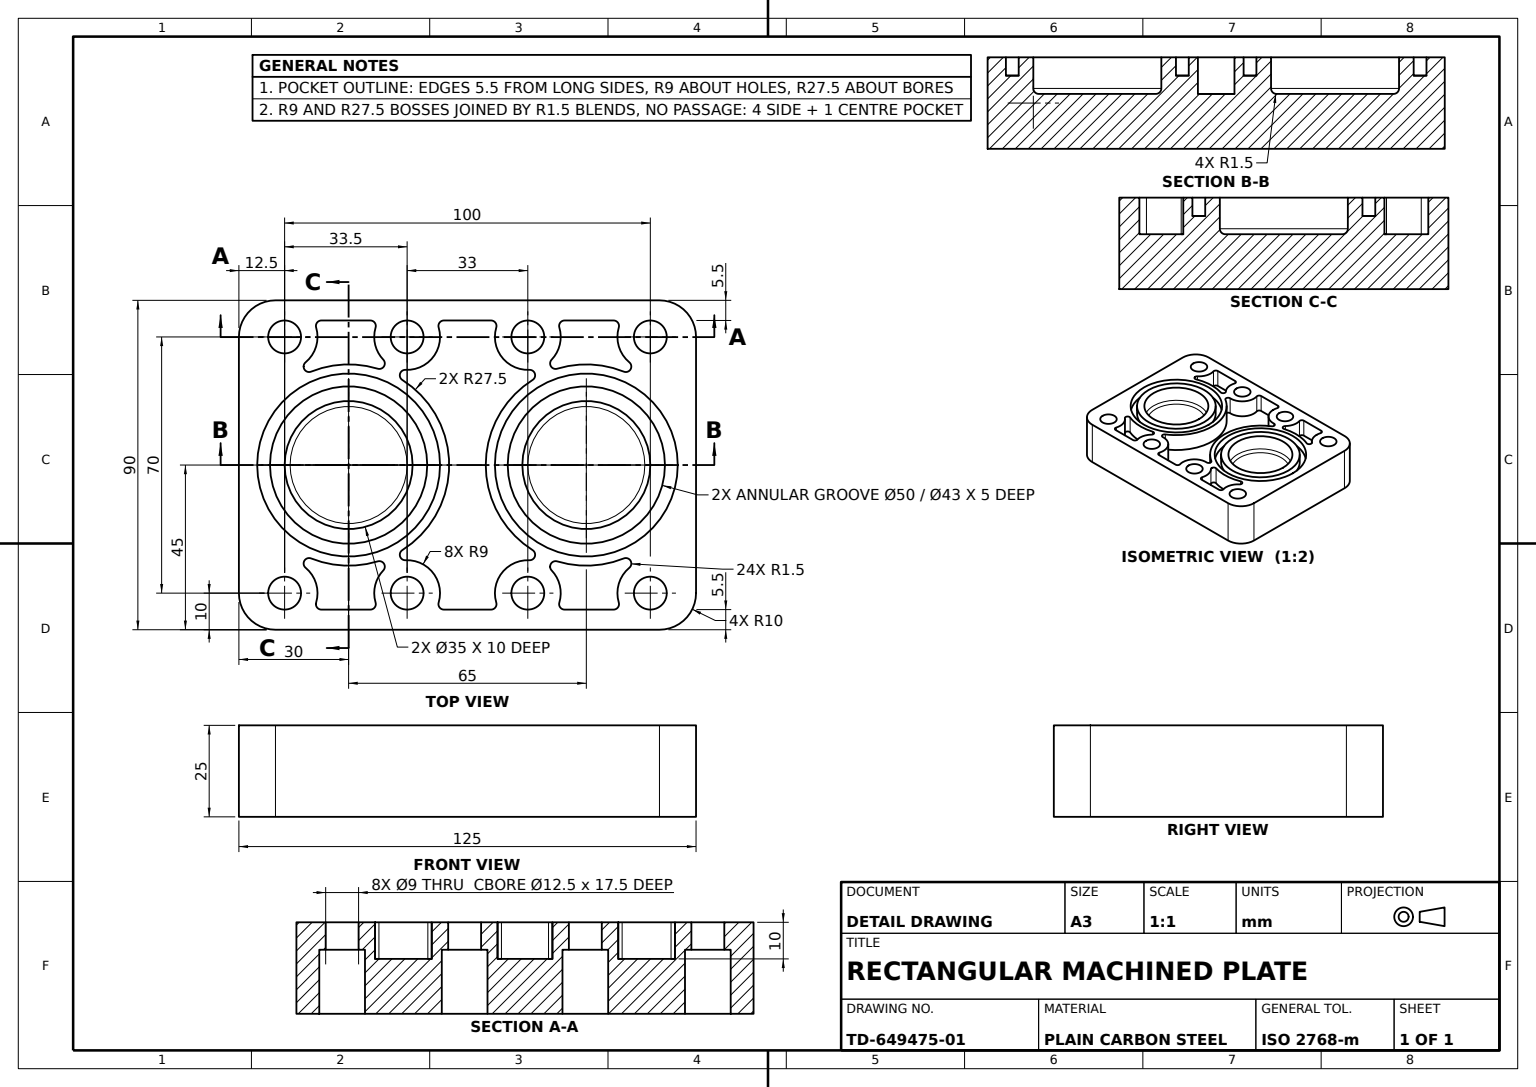
SolidWorks part; units mm, degrees
material "Plain Carbon Steel"
ref_plane "Front Plane" through (0, 0, 0) normal (0, 0, 1) x (1, 0, 0)
ref_plane "Top Plane" through (0, 0, 0) normal (0, 1, 0) x (1, 0, 0)
ref_plane "Right Plane" through (0, 0, 0) normal (1, 0, 0) x (0, 0, -1)
sketch "Block Profile Sketch" plane through (0, 0, 0) normal (1, 0, 0) x (0, 0, -1)
  line L1 (-62.5, 12.5) -> (62.5, 12.5)
  line L2 (-62.5, 12.5) -> (-62.5, -12.5)
  line L3 (-62.5, -12.5) -> (62.5, -12.5)
  line L4 (62.5, 12.5) -> (62.5, -12.5)
  line L5 (-62.5, 12.5) -> (62.5, -12.5) construction
  line L6 (-62.5, -12.5) -> (62.5, 12.5) construction
  point P0 (0, 0)
  dimension "D1" = 25
  dimension "D2" = 125
extrude "Base Block" add sketch "Block Profile Sketch" along normal mid plane 90
sketch "Bore Recess Sketch" plane through (0, 12.5, 0) normal (0, 1, 0) x (1, 0, 0)
  line L0 (0, -62.5) -> (0, 62.5) construction
  line L1 (45, -62.5) -> (-45, -62.5) construction
  line L2 (45, 62.5) -> (-45, 62.5) construction
  line L3 (0, 0) -> (45, 0) construction
  line L4 (45, 62.5) -> (45, -62.5) construction
  circle A0 centre (0, 32.5) radius 25
  circle A1 centre (0, 32.5) radius 21.5
  circle A3 centre (0, -32.5) radius 21.5
  circle A4 centre (0, -32.5) radius 25
  dimension "D1" = 50
  dimension "D2" = 43
  dimension "D3" = 65
extrude "Bore Recess 5mm" cut sketch "Bore Recess Sketch" against normal blind 5
sketch "Twin Bore Sketch" plane through (0, 12.5, 0) normal (0, 1, 0) x (1, 0, 0)
  circle A0 centre (0, 32.5) radius 17.5
  circle A1 centre (0, -32.5) radius 17.5
  dimension "D1" = 35
  dimension "D2" = 35
extrude "Twin Bores" cut sketch "Twin Bore Sketch" against normal blind 10
fillet "Bore Edge Fillet R1.5" radius 1.5 2 edges at (0, 2.5, 50) (0, 2.5, -15)
sketch "Relief Pocket Sketch" plane through (0, 12.5, 0) normal (0, 1, 0) x (1, 0, 0)
  line L0 (-35, 50) -> (-35, -50) construction
  line L1 (0, 0) -> (-45, 0) construction
  line L2 (-45, 62.5) -> (-45, -62.5) construction
  line L3 (-39.5, 6.4377) -> (-39.5, -6.4377)
  line L4 (-39.5, -26.5623) -> (-39.5, -39.9377)
  line L5 (-39.5, 62.5) -> (-39.5, -62.5)
  line L6 (-39.5, 39.9377) -> (-39.5, 26.5623)
  line L7 (0, 0) -> (0, 62.5) construction
  line L8 (45, 62.5) -> (-45, 62.5) construction
  line L9 (39.5, -26.5623) -> (39.5, -39.9377)
  line L10 (39.5, 6.4377) -> (39.5, -6.4377)
  line L11 (39.5, 39.9377) -> (39.5, 26.5623)
  arc A0 (-23.2442, 17.8045) -> (23.2442, 17.8045) centre (0, 32.5) ccw
  arc A1 (-26.3218, -24.5368) -> (-25.5205, -42.7447) centre (0, -32.5) ccw
  arc A2 (-37.5714, 41.3752) -> (-28.0679, 44.2602) centre (-35, 50) ccw
  arc A3 (-37.5714, 7.8752) -> (-26.0103, 16.9311) centre (-35, 16.5) ccw
  arc A4 (-37.5714, -25.1248) -> (-28.7922, -23.0164) centre (-35, -16.5) ccw
  arc A5 (-28.0679, -44.2602) -> (-37.5714, -41.3752) centre (-35, -50) ccw
  arc A6 (-23.2442, 17.8045) -> (-26.0103, 16.9311) centre (-24.5121, 17.0029) ccw
  arc A7 (-25.5205, 42.7447) -> (-28.0679, 44.2602) centre (-26.9125, 43.3035) ccw
  arc A8 (-28.7922, 23.0164) -> (-26.3218, 24.5368) centre (-27.7575, 24.1024) ccw
  arc A9 (-26.3218, -24.5368) -> (-28.7922, -23.0164) centre (-27.7575, -24.1024) ccw
  arc A10 (-28.0679, -44.2602) -> (-25.5205, -42.7447) centre (-26.9125, -43.3035) ccw
  arc A11 (-28.7922, 23.0164) -> (-37.5714, 25.1248) centre (-35, 16.5) ccw
  arc A12 (-37.5714, -41.3752) -> (-39.5, -39.9377) centre (-38, -39.9377) cw
  arc A13 (-37.5714, -25.1248) -> (-39.5, -26.5623) centre (-38, -26.5623) ccw
  arc A14 (-37.5714, 7.8752) -> (-39.5, 6.4377) centre (-38, 6.4377) ccw
  arc A15 (-37.5714, -7.8752) -> (-39.5, -6.4377) centre (-38, -6.4377) cw
  arc A16 (-37.5714, 25.1248) -> (-39.5, 26.5623) centre (-38, 26.5623) cw
  arc A17 (-37.5714, 41.3752) -> (-39.5, 39.9377) centre (-38, 39.9377) ccw
  arc A18 (-26.0103, -16.9311) -> (-23.2442, -17.8045) centre (-24.5121, -17.0029) ccw
  arc A19 (-26.0103, -16.9311) -> (-37.5714, -7.8752) centre (-35, -16.5) ccw
  arc A20 (28.0679, -44.2602) -> (25.5205, -42.7447) centre (26.9125, -43.3035) cw
  arc A21 (28.0679, -44.2602) -> (37.5714, -41.3752) centre (35, -50) cw
  arc A22 (37.5714, -41.3752) -> (39.5, -39.9377) centre (38, -39.9377) ccw
  arc A23 (37.5714, -25.1248) -> (39.5, -26.5623) centre (38, -26.5623) cw
  arc A24 (37.5714, -25.1248) -> (28.7922, -23.0164) centre (35, -16.5) cw
  arc A25 (26.3218, -24.5368) -> (28.7922, -23.0164) centre (27.7575, -24.1024) cw
  arc A26 (26.0103, -16.9311) -> (23.2442, -17.8045) centre (24.5121, -17.0029) cw
  arc A27 (26.0103, -16.9311) -> (37.5714, -7.8752) centre (35, -16.5) cw
  arc A28 (37.5714, -7.8752) -> (39.5, -6.4377) centre (38, -6.4377) ccw
  arc A29 (37.5714, 7.8752) -> (39.5, 6.4377) centre (38, 6.4377) cw
  arc A30 (23.2442, 17.8045) -> (26.0103, 16.9311) centre (24.5121, 17.0029) cw
  arc A31 (37.5714, 7.8752) -> (26.0103, 16.9311) centre (35, 16.5) cw
  arc A32 (37.5714, 41.3752) -> (39.5, 39.9377) centre (38, 39.9377) cw
  arc A33 (37.5714, 25.1248) -> (39.5, 26.5623) centre (38, 26.5623) ccw
  arc A34 (28.7922, 23.0164) -> (26.3218, 24.5368) centre (27.7575, 24.1024) cw
  arc A35 (28.7922, 23.0164) -> (37.5714, 25.1248) centre (35, 16.5) cw
  arc A36 (25.5205, 42.7447) -> (28.0679, 44.2602) centre (26.9125, 43.3035) cw
  arc A37 (37.5714, 41.3752) -> (28.0679, 44.2602) centre (35, 50) cw
  arc A38 (-25.5205, 42.7447) -> (-26.3218, 24.5368) centre (0, 32.5) ccw
  arc A39 (26.3218, 24.5368) -> (25.5205, 42.7447) centre (0, 32.5) ccw
  arc A40 (23.2442, -17.8045) -> (-23.2442, -17.8045) centre (0, -32.5) ccw
  arc A41 (25.5205, -42.7447) -> (26.3218, -24.5368) centre (0, -32.5) ccw
  point P41 (-39.5, -42.2058)
  point P44 (-39.5, -24.2942)
  point P47 (-39.5, 8.7058)
  point P50 (-39.5, -8.7058)
  dimension "D1" = 55
  dimension "D7" = 18
  dimension "D9" = 1.5
  dimension "D10" = 9
  dimension "D11" = 9
  dimension "D12" = 1.5
  dimension "D13" = 9
  dimension "D14" = 27.5
  dimension "D2" = 16.5
  dimension "D3" = 33
  dimension "D4" = 33.5
  dimension "D5" = 33.5
  dimension "D6" = 35
  dimension "D8" = 5.5
extrude "Relief Pockets" cut sketch "Relief Pocket Sketch" against normal blind 10
hole_wizard "Bolt Holes CBore Ø9" positions "Sketch6" profile "Sketch7" legacy
sketch "Sketch6" plane through (0, -12.5, 0) normal (0, -1, 0) x (-1, 0, 0)
  point P0 (-35, -50)
  point P3 (35, -50)
  point P6 (-35, -16.5)
  point P9 (-35, 16.5)
  point P12 (-35, 50)
  point P15 (35, 50)
  point P18 (35, 16.5)
  point P21 (35, -16.5)
sketch "Sketch7" plane through (35, -12.5, 50) normal (1, 0, 0) x (0, 0, -1)
  line L0 (0, 0) -> (0, 100)
  line L1 (0, 100) -> (4.5, 100)
  line L2 (4.5, 100) -> (4.5, 17.5)
  line L3 (4.5, 17.5) -> (6.25, 17.5)
  line L4 (6.25, 17.5) -> (6.25, 0)
  line L5 (6.25, 0) -> (0, 0)
  line L6 (0, 110) -> (0, -10) construction
  dimension "Diameter" = 9
  dimension "Depth" = 100
  dimension "C-Bore Diameter" = 12.5
  dimension "C-Bore Depth" = 17.5
fillet "Corner Fillets R10" radius 10 4 edges at (-45, 0, -62.5) (45, 0, -62.5) (-45, 0, 62.5) (45, 0, 62.5)
